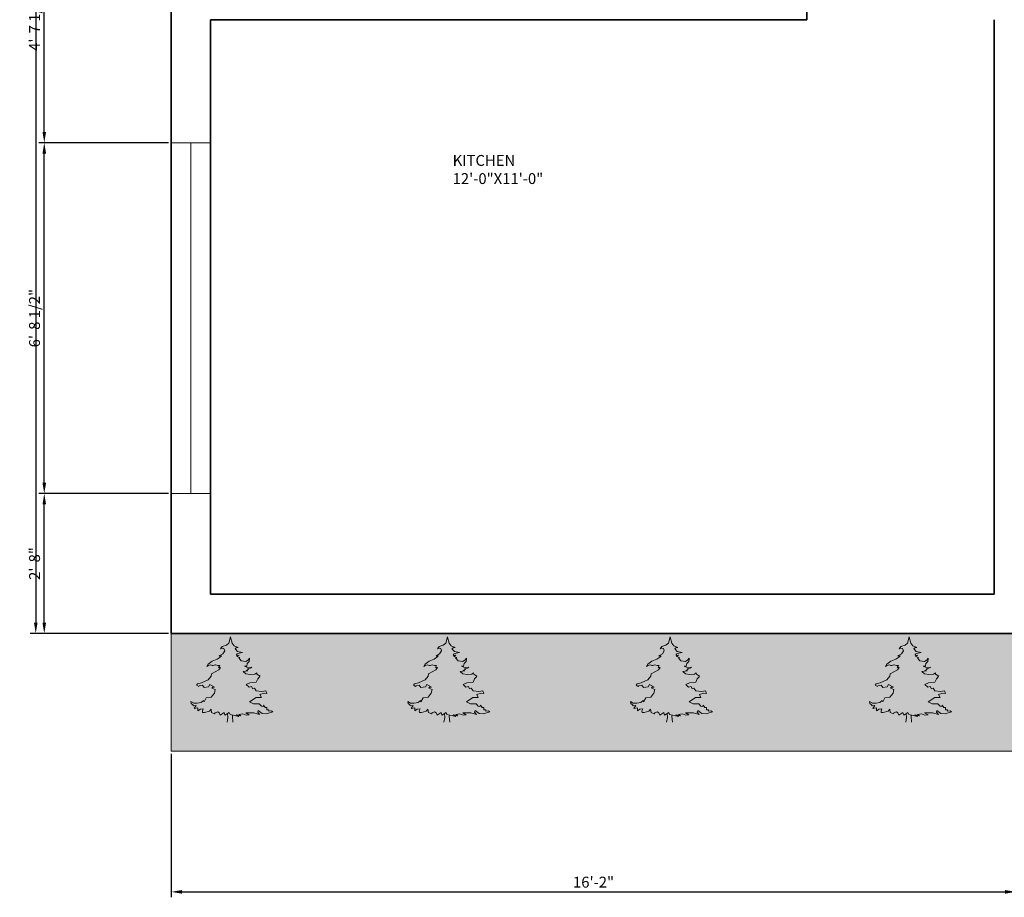
# Model space of a CAD drawing. Units: inches. Extents: x 2981 to 3526, y 1512 to 2158.
# Tile 1 of 4: x 2981 to 3207, y 1512 to 1713. Entities that reach past the tile are written whole.
import ezdxf

# ---------------------------------------------------------------- set-up
doc = ezdxf.new("R2010")
doc.units = ezdxf.units.IN
for name, color, linetype, lineweight in [('A-ANNO-DIMS', 2, 'Continuous', 18), ('A-AREA-IDEN', 7, 'Continuous', 18), ('A-GLAZ', 4, 'Continuous', 18), ('A-WALL', 7, 'Continuous', 35), ('L-GRND-PATT', 8, 'Continuous', 13), ('L-PLNT', 3, 'Continuous', 18), ('L-PLNT-BEDS', 7, 'Continuous', 18)]:
    doc.layers.add(name, color=color, linetype=linetype, lineweight=lineweight)
doc.layers.add('L-PLNT-PATT', color=116, linetype='Continuous', lineweight=13, true_color=0x136734)
doc.styles.get("Standard").update_dxf_attribs({"font": 'arial.ttf'})
doc.dimstyles.new('ISO-25', dxfattribs={"dimtxt": 2.5, "dimasz": 2.5, "dimexe": 1.25, "dimexo": 0.625, "dimtad": 1, "dimlunit": 3, "dimtxsty": 'Standard', "dimcen": 2.5, "dimadec": 0, "dimazin": 0, "dimtfac": 1, "dimtmove": 0, "dimatfit": 3, "dimfxl": 1, "dimarcsym": 0})

# ---------------------------------------------------------------- blocks, each defined once
blk = doc.blocks.new('*U13')
for p, q in [((-9.75, 0), (-8.263, 7.598)), ((-8.263, 7.598), (-8.747, 14.105)), ((-0.771, 9.56), (-0.69, 11.833)), ((0, 0), (-0.771, 9.56))]:
    blk.add_line(p, q)
for points in [[(-3.9, 142.35), (-6.596, 132.037), (-10.801, 128.443), (-17.81, 126.047), (-20.614, 122.452), (-17.81, 123.65), (-15.007, 123.051), (-13.605, 118.858), (-16.876, 114.065), (-21.549, 111.07), (-22.951, 109.872), (-19.212, 110.471), (-19.68, 109.273), (-26.222, 105.079), (-34.633, 101.485), (-41.175, 96.693), (-43.511, 93.098), (-41.175, 94.296), (-36.969, 95.494), (-34.633, 94.296), (-32.764, 94.296), (-29.493, 95.494)], [(-3.759, 141.97), (-1.074, 131.643), (2.437, 127.141), (8.84, 124.493), (6.568, 124.493), (4.09, 123.169), (4.296, 121.846), (7.807, 117.874), (16.069, 116.02), (10.492, 115.226), (5.535, 113.372), (6.981, 112.843), (5.948, 110.989), (10.286, 112.048), (6.775, 109.401), (11.732, 108.077), (9.873, 107.282), (13.797, 102.516), (21.852, 101.192), (25.983, 103.84), (28.048, 106.488), (27.842, 105.164), (27.429, 101.457), (24.124, 97.75), (23.091, 93.513), (19.58, 93.513), (23.505, 91.66), (28.255, 90.866), (31.973, 91.925), (29.081, 89.806), (24.537, 88.747), (26.809, 88.218), (22.472, 86.099), (24.95, 85.57), (17.308, 84.246), (21.852, 80.804), (29.081, 79.215), (36.723, 80.009), (39.821, 82.392), (40.028, 80.009), (45.398, 76.567)], [(-29.25, 95.55), (-25.287, 94.296), (-22.016, 94.296), (-23.885, 91.301), (-20.614, 91.301), (-23.418, 87.108), (-35.567, 80.518), (-36.035, 76.924), (-41.175, 70.334), (-52.389, 65.542), (-58.931, 63.744), (-60.8, 61.348), (-57.062, 59.551), (-56.128, 60.749), (-50.987, 61.348), (-48.184, 57.754), (-40.707, 58.952), (-38.371, 62.546), (-30.427, 58.353), (-33.698, 58.353), (-35.1, 56.556), (-29.493, 54.159), (-30.894, 48.169), (-36.035, 41.579), (-44.446, 40.381), (-48.184, 33.791), (-49.118, 36.188), (-52.857, 32.593), (-59.399, 31.395), (-65.473, 31.395), (-70.146, 34.39), (-69.679, 30.796), (-66.875, 28.999), (-65.941, 27.202), (-61.268, 27.801), (-64.539, 22.409), (-58.464, 23.607), (-58.464, 18.815), (-54.258, 21.211), (-49.586, 21.81), (-50.987, 18.815), (-50.52, 15.82), (-47.249, 15.82), (-39.306, 18.216), (-36.502, 21.211), (-35.567, 15.82), (-30.427, 13.423), (-29.493, 15.221), (-25.287, 17.018), (-22.951, 15.221), (-21.081, 11.626), (-14.539, 15.82), (-13.138, 11.626), (-6.128, 15.82), (-4.726, 12.824), (10.226, 9.23), (5.554, 12.225), (13.497, 10.428), (10.226, 12.824), (16.768, 13.423), (22.376, 11.626), (27.516, 12.225), (21.909, 15.221), (34.993, 15.221), (44.806, 12.824), (41.535, 16.419), (42.469, 19.414), (49.011, 14.023), (56.487, 13.423), (66.768, 17.018), (64.431, 18.815), (60.226, 18.216), (60.226, 20.612), (56.955, 20.612), (56.955, 24.206), (54.151, 24.206), (51.348, 28.4), (50.413, 26.004), (47.609, 26.603), (43.871, 30.197), (38.731, 30.197), (34.525, 30.197), (27.983, 33.791), (38.731, 40.98), (47.609, 40.98), (45.273, 45.773), (52.282, 48.169), (56.955, 47.57), (55.086, 52.362), (48.544, 51.164), (39.198, 52.362), (35.927, 56.556), (33.123, 55.357), (31.254, 59.551), (27.049, 58.353), (22.376, 62.546), (28.451, 65.542), (39.198, 66.74), (41.535, 72.131), (45.273, 76.325)]]:
    blk.add_lwpolyline(points)
blk = doc.blocks.new('*D15')
at = {"layer": 'A-ANNO-DIMS', "color": 0, "lineweight": -2, "transparency": 16777216}
for p, q in [((3014.77, 2112.2), (2983.05, 2112.2)), ((2984.3, 2109.7), (2984.3, 1574.7)), ((3014.77, 1572.2), (2983.05, 1572.2))]:
    blk.add_line(p, q, dxfattribs=at)
at = {"layer": 'A-ANNO-DIMS', "color": 0, "transparency": 16777216}
for points in [[(2983.89, 2109.7), (2984.72, 2109.7), (2984.3, 2112.2)], [(2983.89, 1574.7), (2984.72, 1574.7), (2984.3, 1572.2)]]:
    blk.add_solid(points, dxfattribs=at)
at = {"layer": 'Defpoints', "color": 0, "transparency": 16777216}
for p in [(3015.4, 2112.2), (2984.3, 1572.2), (3015.4, 1572.2)]:
    blk.add_point(p, dxfattribs=at)
at = {"layer": 'A-ANNO-DIMS', "color": 0, "transparency": 16777216, "insert": (2982.41, 1842.2), "char_height": 2.5, "attachment_point": 5, "rotation": 90}
blk.add_mtext("45'", dxfattribs=at)
blk = doc.blocks.new('*D40')
at = {"layer": 'A-ANNO-DIMS', "color": 0, "lineweight": -2, "transparency": 16777216}
for p, q in [((3015.4, 1544.58), (3015.4, 1511.59)), ((3209.4, 1544.58), (3209.4, 1511.59)), ((3017.9, 1512.84), (3206.9, 1512.84))]:
    blk.add_line(p, q, dxfattribs=at)
at = {"layer": 'A-ANNO-DIMS', "color": 0, "transparency": 16777216}
for points in [[(3017.9, 1513.26), (3017.9, 1512.43), (3015.4, 1512.84)], [(3206.9, 1513.26), (3206.9, 1512.43), (3209.4, 1512.84)]]:
    blk.add_solid(points, dxfattribs=at)
at = {"layer": 'Defpoints', "color": 0, "transparency": 16777216}
for p in [(3015.4, 1545.2), (3209.4, 1545.2), (3209.4, 1512.84)]:
    blk.add_point(p, dxfattribs=at)
at = {"layer": 'A-ANNO-DIMS', "color": 0, "transparency": 16777216, "insert": (3112.4, 1514.75), "char_height": 2.5, "attachment_point": 5}
blk.add_mtext('16\'-2"', dxfattribs=at)
blk = doc.blocks.new('*D44')
at = {"layer": 'A-ANNO-DIMS', "color": 0, "lineweight": -2, "transparency": 16777216}
for p, q in [((3014.77, 1684.94), (2985, 1684.94)), ((2986.25, 1606.84), (2986.25, 1682.44)), ((3014.77, 1604.34), (2985, 1604.34))]:
    blk.add_line(p, q, dxfattribs=at)
at = {"layer": 'A-ANNO-DIMS', "color": 0, "transparency": 16777216}
for points in [[(2985.84, 1682.44), (2986.67, 1682.44), (2986.25, 1684.94)], [(2985.84, 1606.84), (2986.67, 1606.84), (2986.25, 1604.34)]]:
    blk.add_solid(points, dxfattribs=at)
at = {"layer": 'Defpoints', "color": 0, "transparency": 16777216}
for p in [(2986.25, 1684.94), (3015.4, 1684.94), (3015.4, 1604.34)]:
    blk.add_point(p, dxfattribs=at)
at = {"layer": 'A-ANNO-DIMS', "color": 0, "transparency": 16777216, "insert": (2984.34, 1644.64), "char_height": 2.5, "attachment_point": 5, "rotation": 90}
blk.add_mtext('6\'-8 1/2"', dxfattribs=at)
blk = doc.blocks.new('*D45')
at = {"layer": 'A-ANNO-DIMS', "color": 0, "lineweight": -2, "transparency": 16777216}
for p, q in [((3014.77, 1604.34), (2985, 1604.34)), ((2986.25, 1574.7), (2986.25, 1601.84)), ((3014.77, 1572.2), (2985, 1572.2))]:
    blk.add_line(p, q, dxfattribs=at)
at = {"layer": 'A-ANNO-DIMS', "color": 0, "transparency": 16777216}
for points in [[(2985.84, 1601.84), (2986.67, 1601.84), (2986.25, 1604.34)], [(2985.84, 1574.7), (2986.67, 1574.7), (2986.25, 1572.2)]]:
    blk.add_solid(points, dxfattribs=at)
at = {"layer": 'Defpoints', "color": 0, "transparency": 16777216}
for p in [(2986.25, 1604.34), (3015.4, 1604.34), (3015.4, 1572.2)]:
    blk.add_point(p, dxfattribs=at)
at = {"layer": 'A-ANNO-DIMS', "color": 0, "transparency": 16777216, "insert": (2984.35, 1588.27), "char_height": 2.5, "attachment_point": 5, "rotation": 90}
blk.add_mtext('2\'-8"', dxfattribs=at)
blk = doc.blocks.new('*D51')
at = {"layer": 'A-ANNO-DIMS', "color": 0, "lineweight": -2, "transparency": 16777216}
for p, q in [((3014.77, 1740.56), (2985, 1740.56)), ((2986.25, 1687.44), (2986.25, 1738.06)), ((3014.77, 1684.94), (2985, 1684.94))]:
    blk.add_line(p, q, dxfattribs=at)
at = {"layer": 'A-ANNO-DIMS', "color": 0, "transparency": 16777216}
for points in [[(2985.84, 1738.06), (2986.67, 1738.06), (2986.25, 1740.56)], [(2985.84, 1687.44), (2986.67, 1687.44), (2986.25, 1684.94)]]:
    blk.add_solid(points, dxfattribs=at)
at = {"layer": 'Defpoints', "color": 0, "transparency": 16777216}
for p in [(2986.25, 1740.56), (3015.4, 1740.56), (3015.4, 1684.94)]:
    blk.add_point(p, dxfattribs=at)
at = {"layer": 'A-ANNO-DIMS', "color": 0, "transparency": 16777216, "insert": (2984.34, 1712.75), "char_height": 2.5, "attachment_point": 5, "rotation": 90}
blk.add_mtext('4\'-7 1/2"', dxfattribs=at)

msp = doc.modelspace()

# ---------------------------------------------------------------- hatches: boundary and pattern name
at = {"layer": 'L-GRND-PATT'}
h = msp.add_hatch(color=256, dxfattribs=at)
h.dxf.hatch_style = 1
h.paths.add_polyline_path([(3209.399, 1563.202), (3209.399, 1572.202), (3015.399, 1572.202), (3015.399, 1545.202), (3209.399, 1545.202), (3209.399, 1554.202)])
h.paths.add_polyline_path([(3038.736, 1554.203), (3037.324, 1553.709), (3036.297, 1553.792), (3035.398, 1554.532), (3035.27, 1554.121), (3035.719, 1553.627), (3034.371, 1553.956), (3032.573, 1553.956), (3033.344, 1553.545), (3032.638, 1553.462), (3031.867, 1553.709), (3030.968, 1553.627), (3031.418, 1553.298), (3030.327, 1553.545), (3030.968, 1553.133), (3028.914, 1553.627), (3028.722, 1554.039), (3027.759, 1553.462), (3027.566, 1554.039), (3026.668, 1553.462), (3026.411, 1553.956), (3026.09, 1554.203), (3025.512, 1553.956), (3025.384, 1553.709), (3024.677, 1554.039), (3024.549, 1554.779), (3024.164, 1554.368), (3023.073, 1554.039), (3022.623, 1554.039), (3022.559, 1554.45), (3022.752, 1554.861), (3022.11, 1554.779), (3021.532, 1554.45), (3021.532, 1555.108), (3020.697, 1554.944), (3021.147, 1555.684), (3020.505, 1555.602), (3020.376, 1555.849), (3019.991, 1556.096), (3019.927, 1556.59), (3020.569, 1556.178), (3021.403, 1556.178), (3022.302, 1556.343), (3022.816, 1556.837), (3022.944, 1556.507), (3023.458, 1557.413), (3024.613, 1557.577), (3025.319, 1558.483), (3025.512, 1559.306), (3024.742, 1559.635), (3024.934, 1559.882), (3025.384, 1559.882), (3024.292, 1560.458), (3023.971, 1559.964), (3022.944, 1559.799), (3022.559, 1560.293), (3021.853, 1560.211), (3021.724, 1560.046), (3021.211, 1560.293), (3021.468, 1560.622), (3022.366, 1560.869), (3023.907, 1561.528), (3024.613, 1562.433), (3024.677, 1562.927), (3026.346, 1563.832), (3026.732, 1564.408), (3026.282, 1564.408), (3026.539, 1564.82), (3026.09, 1564.82), (3025.539, 1564.994), (3024.913, 1564.765), (3024.485, 1564.984), (3023.907, 1564.82), (3023.586, 1564.655), (3023.907, 1565.149), (3024.806, 1565.807), (3025.961, 1566.301), (3026.86, 1566.877), (3026.924, 1567.042), (3026.411, 1566.959), (3026.603, 1567.124), (3027.245, 1567.535), (3027.695, 1568.194), (3027.502, 1568.77), (3027.117, 1568.852), (3026.732, 1568.688), (3027.117, 1569.181), (3028.08, 1569.511), (3028.657, 1570.004), (3029.031, 1571.432), (3029.416, 1569.95), (3029.898, 1569.332), (3030.778, 1568.968), (3030.466, 1568.968), (3030.126, 1568.786), (3030.154, 1568.604), (3030.636, 1568.059), (3031.771, 1567.804), (3031.005, 1567.695), (3030.324, 1567.44), (3030.523, 1567.368), (3030.381, 1567.113), (3030.977, 1567.258), (3030.494, 1566.895), (3031.175, 1566.713), (3030.92, 1566.604), (3031.459, 1565.949), (3032.566, 1565.767), (3033.133, 1566.131), (3033.417, 1566.494), (3033.389, 1566.313), (3033.332, 1565.803), (3032.878, 1565.294), (3032.736, 1564.712), (3032.254, 1564.712), (3032.793, 1564.457), (3033.445, 1564.348), (3033.956, 1564.494), (3033.559, 1564.203), (3032.935, 1564.057), (3033.247, 1563.985), (3032.651, 1563.693), (3032.991, 1563.621), (3031.941, 1563.439), (3032.566, 1562.966), (3033.559, 1562.748), (3034.609, 1562.857), (3035.034, 1563.184), (3035.063, 1562.857), (3035.808, 1562.379), (3035.27, 1561.775), (3034.949, 1561.034), (3033.472, 1560.869), (3032.638, 1560.458), (3033.28, 1559.882), (3033.857, 1560.046), (3034.114, 1559.47), (3034.499, 1559.635), (3034.949, 1559.059), (3036.233, 1558.894), (3037.131, 1559.059), (3037.388, 1558.4), (3036.746, 1558.483), (3035.783, 1558.153), (3036.104, 1557.495), (3034.884, 1557.495), (3033.408, 1556.507), (3034.307, 1556.014), (3034.884, 1556.014), (3035.591, 1556.014), (3036.104, 1555.52), (3036.489, 1555.438), (3036.618, 1555.767), (3037.003, 1555.191), (3037.388, 1555.191), (3037.388, 1554.697), (3037.837, 1554.697), (3037.837, 1554.368), (3038.415, 1554.45)], flags=16)
h.paths.add_polyline_path([(3069.74, 1556.59), (3070.382, 1556.178), (3071.217, 1556.178), (3072.115, 1556.343), (3072.629, 1556.837), (3072.757, 1556.507), (3073.271, 1557.413), (3074.426, 1557.577), (3075.133, 1558.483), (3075.325, 1559.306), (3074.555, 1559.635), (3074.747, 1559.882), (3075.197, 1559.882), (3074.105, 1560.458), (3073.785, 1559.964), (3072.757, 1559.799), (3072.372, 1560.293), (3071.666, 1560.211), (3071.538, 1560.046), (3071.024, 1560.293), (3071.281, 1560.622), (3072.18, 1560.869), (3073.72, 1561.528), (3074.426, 1562.433), (3074.491, 1562.927), (3076.16, 1563.832), (3076.545, 1564.408), (3076.096, 1564.408), (3076.352, 1564.82), (3075.903, 1564.82), (3075.352, 1564.994), (3074.726, 1564.765), (3074.298, 1564.984), (3073.72, 1564.82), (3073.399, 1564.655), (3073.72, 1565.149), (3074.619, 1565.807), (3075.774, 1566.301), (3076.673, 1566.877), (3076.737, 1567.042), (3076.224, 1566.959), (3076.416, 1567.124), (3077.058, 1567.535), (3077.508, 1568.194), (3077.315, 1568.77), (3076.93, 1568.852), (3076.545, 1568.688), (3076.93, 1569.181), (3077.893, 1569.511), (3078.471, 1570.004), (3078.844, 1571.432), (3079.229, 1569.95), (3079.712, 1569.332), (3080.591, 1568.968), (3080.279, 1568.968), (3079.939, 1568.786), (3079.967, 1568.604), (3080.449, 1568.059), (3081.584, 1567.804), (3080.818, 1567.695), (3080.137, 1567.44), (3080.336, 1567.368), (3080.194, 1567.113), (3080.79, 1567.258), (3080.308, 1566.895), (3080.989, 1566.713), (3080.733, 1566.604), (3081.272, 1565.949), (3082.379, 1565.767), (3082.946, 1566.131), (3083.23, 1566.494), (3083.202, 1566.313), (3083.145, 1565.803), (3082.691, 1565.294), (3082.549, 1564.712), (3082.067, 1564.712), (3082.606, 1564.457), (3083.258, 1564.348), (3083.769, 1564.494), (3083.372, 1564.203), (3082.748, 1564.057), (3083.06, 1563.985), (3082.464, 1563.693), (3082.804, 1563.621), (3081.755, 1563.439), (3082.379, 1562.966), (3083.372, 1562.748), (3084.422, 1562.857), (3084.847, 1563.184), (3084.876, 1562.857), (3085.622, 1562.379), (3085.083, 1561.775), (3084.762, 1561.034), (3083.285, 1560.869), (3082.451, 1560.458), (3083.093, 1559.882), (3083.67, 1560.046), (3083.927, 1559.47), (3084.312, 1559.635), (3084.762, 1559.059), (3086.046, 1558.894), (3086.945, 1559.059), (3087.201, 1558.4), (3086.559, 1558.483), (3085.596, 1558.153), (3085.917, 1557.495), (3084.698, 1557.495), (3083.221, 1556.507), (3084.12, 1556.014), (3084.698, 1556.014), (3085.404, 1556.014), (3085.917, 1555.52), (3086.303, 1555.438), (3086.431, 1555.767), (3086.816, 1555.191), (3087.201, 1555.191), (3087.201, 1554.697), (3087.651, 1554.697), (3087.651, 1554.368), (3088.228, 1554.45), (3088.549, 1554.203), (3087.137, 1553.709), (3086.11, 1553.792), (3085.211, 1554.532), (3085.083, 1554.121), (3085.532, 1553.627), (3084.184, 1553.956), (3082.387, 1553.956), (3083.157, 1553.545), (3082.451, 1553.462), (3081.68, 1553.709), (3080.782, 1553.627), (3081.231, 1553.298), (3080.14, 1553.545), (3080.782, 1553.133), (3078.728, 1553.627), (3078.535, 1554.039), (3077.572, 1553.462), (3077.379, 1554.039), (3076.481, 1553.462), (3076.224, 1553.956), (3075.903, 1554.203), (3075.325, 1553.956), (3075.197, 1553.709), (3074.491, 1554.039), (3074.362, 1554.779), (3073.977, 1554.368), (3072.886, 1554.039), (3072.436, 1554.039), (3072.372, 1554.45), (3072.565, 1554.861), (3071.923, 1554.779), (3071.345, 1554.45), (3071.345, 1555.108), (3070.51, 1554.944), (3070.96, 1555.684), (3070.318, 1555.602), (3070.19, 1555.849), (3069.804, 1556.096)], flags=16)
h.paths.add_polyline_path([(3120.884, 1556.59), (3121.526, 1556.178), (3122.361, 1556.178), (3123.259, 1556.343), (3123.773, 1556.837), (3123.901, 1556.507), (3124.415, 1557.413), (3125.57, 1557.577), (3126.277, 1558.483), (3126.469, 1559.306), (3125.699, 1559.635), (3125.891, 1559.882), (3126.341, 1559.882), (3125.249, 1560.458), (3124.928, 1559.964), (3123.901, 1559.799), (3123.516, 1560.293), (3122.81, 1560.211), (3122.682, 1560.046), (3122.168, 1560.293), (3122.425, 1560.622), (3123.324, 1560.869), (3124.864, 1561.528), (3125.57, 1562.433), (3125.635, 1562.927), (3127.304, 1563.832), (3127.689, 1564.408), (3127.239, 1564.408), (3127.496, 1564.82), (3127.047, 1564.82), (3126.496, 1564.994), (3125.87, 1564.765), (3125.442, 1564.984), (3124.864, 1564.82), (3124.543, 1564.655), (3124.864, 1565.149), (3125.763, 1565.807), (3126.918, 1566.301), (3127.817, 1566.877), (3127.881, 1567.042), (3127.368, 1566.959), (3127.56, 1567.124), (3128.202, 1567.535), (3128.652, 1568.194), (3128.459, 1568.77), (3128.074, 1568.852), (3127.689, 1568.688), (3128.074, 1569.181), (3129.037, 1569.511), (3129.615, 1570.004), (3129.988, 1571.432), (3130.373, 1569.95), (3130.856, 1569.332), (3131.735, 1568.968), (3131.423, 1568.968), (3131.083, 1568.786), (3131.111, 1568.604), (3131.593, 1568.059), (3132.728, 1567.804), (3131.962, 1567.695), (3131.281, 1567.44), (3131.48, 1567.368), (3131.338, 1567.113), (3131.934, 1567.258), (3131.452, 1566.895), (3132.133, 1566.713), (3131.877, 1566.604), (3132.416, 1565.949), (3133.523, 1565.767), (3134.09, 1566.131), (3134.374, 1566.494), (3134.346, 1566.313), (3134.289, 1565.803), (3133.835, 1565.294), (3133.693, 1564.712), (3133.211, 1564.712), (3133.75, 1564.457), (3134.402, 1564.348), (3134.913, 1564.494), (3134.516, 1564.203), (3133.892, 1564.057), (3134.204, 1563.985), (3133.608, 1563.693), (3133.948, 1563.621), (3132.899, 1563.439), (3133.523, 1562.966), (3134.516, 1562.748), (3135.566, 1562.857), (3135.991, 1563.184), (3136.02, 1562.857), (3136.765, 1562.379), (3136.227, 1561.775), (3135.906, 1561.034), (3134.429, 1560.869), (3133.595, 1560.458), (3134.237, 1559.882), (3134.814, 1560.046), (3135.071, 1559.47), (3135.456, 1559.635), (3135.906, 1559.059), (3137.19, 1558.894), (3138.088, 1559.059), (3138.345, 1558.4), (3137.703, 1558.483), (3136.74, 1558.153), (3137.061, 1557.495), (3135.842, 1557.495), (3134.365, 1556.507), (3135.264, 1556.014), (3135.842, 1556.014), (3136.548, 1556.014), (3137.061, 1555.52), (3137.446, 1555.438), (3137.575, 1555.767), (3137.96, 1555.191), (3138.345, 1555.191), (3138.345, 1554.697), (3138.795, 1554.697), (3138.795, 1554.368), (3139.372, 1554.45), (3139.693, 1554.203), (3138.281, 1553.709), (3137.254, 1553.792), (3136.355, 1554.532), (3136.227, 1554.121), (3136.676, 1553.627), (3135.328, 1553.956), (3133.531, 1553.956), (3134.301, 1553.545), (3133.595, 1553.462), (3132.824, 1553.709), (3131.926, 1553.627), (3132.375, 1553.298), (3131.284, 1553.545), (3131.926, 1553.133), (3129.872, 1553.627), (3129.679, 1554.039), (3128.716, 1553.462), (3128.523, 1554.039), (3127.625, 1553.462), (3127.368, 1553.956), (3127.047, 1554.203), (3126.469, 1553.956), (3126.341, 1553.709), (3125.635, 1554.039), (3125.506, 1554.779), (3125.121, 1554.368), (3124.03, 1554.039), (3123.58, 1554.039), (3123.516, 1554.45), (3123.709, 1554.861), (3123.067, 1554.779), (3122.489, 1554.45), (3122.489, 1555.108), (3121.654, 1554.944), (3122.104, 1555.684), (3121.462, 1555.602), (3121.334, 1555.849), (3120.948, 1556.096)], flags=16)
h.paths.add_polyline_path([(3175.793, 1556.59), (3176.435, 1556.178), (3177.27, 1556.178), (3178.169, 1556.343), (3178.682, 1556.837), (3178.811, 1556.507), (3179.324, 1557.413), (3180.48, 1557.577), (3181.186, 1558.483), (3181.378, 1559.306), (3180.608, 1559.635), (3180.801, 1559.882), (3181.25, 1559.882), (3180.159, 1560.458), (3179.838, 1559.964), (3178.811, 1559.799), (3178.425, 1560.293), (3177.719, 1560.211), (3177.591, 1560.046), (3177.077, 1560.293), (3177.334, 1560.622), (3178.233, 1560.869), (3179.773, 1561.528), (3180.48, 1562.433), (3180.544, 1562.927), (3182.213, 1563.832), (3182.598, 1564.408), (3182.149, 1564.408), (3182.406, 1564.82), (3181.956, 1564.82), (3181.405, 1564.994), (3180.779, 1564.765), (3180.351, 1564.984), (3179.773, 1564.82), (3179.453, 1564.655), (3179.773, 1565.149), (3180.672, 1565.807), (3181.828, 1566.301), (3182.726, 1566.877), (3182.791, 1567.042), (3182.277, 1566.959), (3182.47, 1567.124), (3183.112, 1567.535), (3183.561, 1568.194), (3183.368, 1568.77), (3182.983, 1568.852), (3182.598, 1568.688), (3182.983, 1569.181), (3183.946, 1569.511), (3184.524, 1570.004), (3184.897, 1571.432), (3185.283, 1569.95), (3185.765, 1569.332), (3186.645, 1568.968), (3186.332, 1568.968), (3185.992, 1568.786), (3186.02, 1568.604), (3186.503, 1568.059), (3187.638, 1567.804), (3186.871, 1567.695), (3186.19, 1567.44), (3186.389, 1567.368), (3186.247, 1567.113), (3186.843, 1567.258), (3186.361, 1566.895), (3187.042, 1566.713), (3186.786, 1566.604), (3187.325, 1565.949), (3188.432, 1565.767), (3189, 1566.131), (3189.283, 1566.494), (3189.255, 1566.313), (3189.198, 1565.803), (3188.744, 1565.294), (3188.602, 1564.712), (3188.12, 1564.712), (3188.659, 1564.457), (3189.312, 1564.348), (3189.823, 1564.494), (3189.425, 1564.203), (3188.801, 1564.057), (3189.113, 1563.985), (3188.517, 1563.693), (3188.858, 1563.621), (3187.808, 1563.439), (3188.432, 1562.966), (3189.425, 1562.748), (3190.475, 1562.857), (3190.901, 1563.184), (3190.929, 1562.857), (3191.675, 1562.379), (3191.136, 1561.775), (3190.815, 1561.034), (3189.339, 1560.869), (3188.504, 1560.458), (3189.146, 1559.882), (3189.724, 1560.046), (3189.98, 1559.47), (3190.366, 1559.635), (3190.815, 1559.059), (3192.099, 1558.894), (3192.998, 1559.059), (3193.255, 1558.4), (3192.613, 1558.483), (3191.65, 1558.153), (3191.971, 1557.495), (3190.751, 1557.495), (3189.274, 1556.507), (3190.173, 1556.014), (3190.751, 1556.014), (3191.457, 1556.014), (3191.971, 1555.52), (3192.356, 1555.438), (3192.484, 1555.767), (3192.869, 1555.191), (3193.255, 1555.191), (3193.255, 1554.697), (3193.704, 1554.697), (3193.704, 1554.368), (3194.282, 1554.45), (3194.603, 1554.203), (3193.19, 1553.709), (3192.163, 1553.792), (3191.264, 1554.532), (3191.136, 1554.121), (3191.586, 1553.627), (3190.237, 1553.956), (3188.44, 1553.956), (3189.21, 1553.545), (3188.504, 1553.462), (3187.734, 1553.709), (3186.835, 1553.627), (3187.284, 1553.298), (3186.193, 1553.545), (3186.835, 1553.133), (3184.781, 1553.627), (3184.588, 1554.039), (3183.625, 1553.462), (3183.433, 1554.039), (3182.534, 1553.462), (3182.277, 1553.956), (3181.956, 1554.203), (3181.378, 1553.956), (3181.25, 1553.709), (3180.544, 1554.039), (3180.415, 1554.779), (3180.03, 1554.368), (3178.939, 1554.039), (3178.49, 1554.039), (3178.425, 1554.45), (3178.618, 1554.861), (3177.976, 1554.779), (3177.398, 1554.45), (3177.398, 1555.108), (3176.564, 1554.944), (3177.013, 1555.684), (3176.371, 1555.602), (3176.243, 1555.849), (3175.858, 1556.096)], flags=16)
at = {"layer": 'L-PLNT-PATT'}
h = msp.add_hatch(color=256, dxfattribs=at)
h.dxf.hatch_style = 1
h.paths.add_polyline_path([(3035.808, 1562.379), (3035.063, 1562.857), (3035.034, 1563.184), (3034.609, 1562.857), (3033.559, 1562.748), (3032.566, 1562.966), (3031.941, 1563.439), (3032.991, 1563.621), (3032.651, 1563.693), (3033.247, 1563.985), (3032.935, 1564.057), (3033.559, 1564.203), (3033.956, 1564.494), (3033.445, 1564.348), (3032.793, 1564.457), (3032.254, 1564.712), (3032.736, 1564.712), (3032.878, 1565.294), (3033.332, 1565.803), (3033.407, 1566.482), (3033.133, 1566.131), (3032.566, 1565.767), (3031.459, 1565.949), (3030.92, 1566.604), (3031.175, 1566.713), (3030.494, 1566.895), (3030.977, 1567.258), (3030.381, 1567.113), (3030.523, 1567.368), (3030.324, 1567.44), (3031.005, 1567.695), (3031.771, 1567.804), (3030.636, 1568.059), (3030.036, 1568.738), (3030.602, 1569.041), (3029.898, 1569.332), (3029.416, 1569.95), (3029.031, 1571.432), (3028.657, 1570.004), (3028.08, 1569.511), (3027.117, 1569.181), (3026.732, 1568.688), (3027.117, 1568.852), (3027.502, 1568.77), (3027.695, 1568.194), (3027.245, 1567.535), (3026.603, 1567.124), (3026.411, 1566.959), (3026.924, 1567.042), (3026.86, 1566.877), (3025.961, 1566.301), (3024.806, 1565.807), (3023.907, 1565.149), (3023.586, 1564.655), (3023.907, 1564.82), (3024.485, 1564.984), (3024.806, 1564.82), (3025.063, 1564.82), (3025.539, 1564.994), (3026.09, 1564.82), (3026.539, 1564.82), (3026.282, 1564.408), (3026.732, 1564.408), (3026.346, 1563.832), (3024.677, 1562.927), (3024.613, 1562.433), (3023.907, 1561.528), (3022.366, 1560.869), (3021.468, 1560.622), (3021.211, 1560.293), (3021.724, 1560.046), (3021.853, 1560.211), (3022.559, 1560.293), (3022.944, 1559.799), (3023.971, 1559.964), (3024.292, 1560.458), (3025.384, 1559.882), (3024.934, 1559.882), (3024.742, 1559.635), (3025.512, 1559.306), (3025.319, 1558.483), (3024.613, 1557.577), (3023.458, 1557.413), (3022.944, 1556.507), (3022.816, 1556.837), (3022.302, 1556.343), (3021.403, 1556.178), (3020.569, 1556.178), (3019.927, 1556.59), (3019.991, 1556.096), (3020.376, 1555.849), (3020.505, 1555.602), (3021.147, 1555.684), (3020.697, 1554.944), (3021.532, 1555.108), (3021.532, 1554.45), (3022.11, 1554.779), (3022.752, 1554.861), (3022.559, 1554.45), (3022.623, 1554.039), (3023.073, 1554.039), (3024.164, 1554.368), (3024.549, 1554.779), (3024.677, 1554.039), (3025.384, 1553.709), (3025.512, 1553.956), (3026.09, 1554.203), (3026.411, 1553.956), (3026.668, 1553.462), (3027.566, 1554.039), (3027.759, 1553.462), (3028.722, 1554.039), (3028.914, 1553.627), (3030.968, 1553.133), (3030.327, 1553.545), (3031.418, 1553.298), (3030.968, 1553.627), (3031.867, 1553.709), (3032.638, 1553.462), (3033.344, 1553.545), (3032.573, 1553.956), (3034.371, 1553.956), (3035.719, 1553.627), (3035.27, 1554.121), (3035.398, 1554.532), (3036.297, 1553.792), (3037.324, 1553.709), (3038.736, 1554.203), (3038.415, 1554.45), (3037.837, 1554.368), (3037.837, 1554.697), (3037.388, 1554.697), (3037.388, 1555.191), (3037.003, 1555.191), (3036.618, 1555.767), (3036.489, 1555.438), (3036.104, 1555.52), (3035.591, 1556.014), (3034.884, 1556.014), (3034.307, 1556.014), (3033.408, 1556.507), (3034.884, 1557.495), (3036.104, 1557.495), (3035.783, 1558.153), (3036.746, 1558.483), (3037.388, 1558.4), (3037.131, 1559.059), (3036.233, 1558.894), (3034.949, 1559.059), (3034.499, 1559.635), (3034.114, 1559.47), (3033.857, 1560.046), (3033.28, 1559.882), (3032.638, 1560.458), (3033.472, 1560.869), (3034.949, 1561.034), (3035.27, 1561.775)])
h.paths.add_polyline_path([(3084.312, 1559.635), (3083.927, 1559.47), (3083.67, 1560.046), (3083.093, 1559.882), (3082.451, 1560.458), (3083.285, 1560.869), (3084.762, 1561.034), (3085.083, 1561.775), (3085.622, 1562.379), (3084.876, 1562.857), (3084.847, 1563.184), (3084.422, 1562.857), (3083.372, 1562.748), (3082.379, 1562.966), (3081.755, 1563.439), (3082.804, 1563.621), (3082.464, 1563.693), (3083.06, 1563.985), (3082.748, 1564.057), (3083.372, 1564.203), (3083.769, 1564.494), (3083.258, 1564.348), (3082.606, 1564.457), (3082.067, 1564.712), (3082.549, 1564.712), (3082.691, 1565.294), (3083.145, 1565.803), (3083.221, 1566.482), (3082.946, 1566.131), (3082.379, 1565.767), (3081.272, 1565.949), (3080.733, 1566.604), (3080.989, 1566.713), (3080.308, 1566.895), (3080.79, 1567.258), (3080.194, 1567.113), (3080.336, 1567.368), (3080.137, 1567.44), (3080.818, 1567.695), (3081.584, 1567.804), (3080.449, 1568.059), (3079.849, 1568.738), (3080.415, 1569.041), (3079.712, 1569.332), (3079.229, 1569.95), (3078.844, 1571.432), (3078.471, 1570.004), (3077.893, 1569.511), (3076.93, 1569.181), (3076.545, 1568.688), (3076.93, 1568.852), (3077.315, 1568.77), (3077.508, 1568.194), (3077.058, 1567.535), (3076.416, 1567.124), (3076.224, 1566.959), (3076.737, 1567.042), (3076.673, 1566.877), (3075.774, 1566.301), (3074.619, 1565.807), (3073.72, 1565.149), (3073.399, 1564.655), (3073.72, 1564.82), (3074.298, 1564.984), (3074.619, 1564.82), (3074.876, 1564.82), (3075.352, 1564.994), (3075.903, 1564.82), (3076.352, 1564.82), (3076.096, 1564.408), (3076.545, 1564.408), (3076.16, 1563.832), (3074.491, 1562.927), (3074.426, 1562.433), (3073.72, 1561.528), (3072.18, 1560.869), (3071.281, 1560.622), (3071.024, 1560.293), (3071.538, 1560.046), (3071.666, 1560.211), (3072.372, 1560.293), (3072.757, 1559.799), (3073.785, 1559.964), (3074.105, 1560.458), (3075.197, 1559.882), (3074.747, 1559.882), (3074.555, 1559.635), (3075.325, 1559.306), (3075.133, 1558.483), (3074.426, 1557.577), (3073.271, 1557.413), (3072.757, 1556.507), (3072.629, 1556.837), (3072.115, 1556.343), (3071.217, 1556.178), (3070.382, 1556.178), (3069.74, 1556.59), (3069.804, 1556.096), (3070.19, 1555.849), (3070.318, 1555.602), (3070.96, 1555.684), (3070.51, 1554.944), (3071.345, 1555.108), (3071.345, 1554.45), (3071.923, 1554.779), (3072.565, 1554.861), (3072.372, 1554.45), (3072.436, 1554.039), (3072.886, 1554.039), (3073.977, 1554.368), (3074.362, 1554.779), (3074.491, 1554.039), (3075.197, 1553.709), (3075.325, 1553.956), (3075.903, 1554.203), (3076.224, 1553.956), (3076.481, 1553.462), (3077.379, 1554.039), (3077.572, 1553.462), (3078.535, 1554.039), (3078.728, 1553.627), (3080.782, 1553.133), (3080.14, 1553.545), (3081.231, 1553.298), (3080.782, 1553.627), (3081.68, 1553.709), (3082.451, 1553.462), (3083.157, 1553.545), (3082.387, 1553.956), (3084.184, 1553.956), (3085.532, 1553.627), (3085.083, 1554.121), (3085.211, 1554.532), (3086.11, 1553.792), (3087.137, 1553.709), (3088.549, 1554.203), (3088.228, 1554.45), (3087.651, 1554.368), (3087.651, 1554.697), (3087.201, 1554.697), (3087.201, 1555.191), (3086.816, 1555.191), (3086.431, 1555.767), (3086.303, 1555.438), (3085.917, 1555.52), (3085.404, 1556.014), (3084.698, 1556.014), (3084.12, 1556.014), (3083.221, 1556.507), (3084.698, 1557.495), (3085.917, 1557.495), (3085.596, 1558.153), (3086.559, 1558.483), (3087.201, 1558.4), (3086.945, 1559.059), (3086.046, 1558.894), (3084.762, 1559.059)])
h.paths.add_polyline_path([(3135.842, 1557.495), (3137.061, 1557.495), (3136.74, 1558.153), (3137.703, 1558.483), (3138.345, 1558.4), (3138.088, 1559.059), (3137.19, 1558.894), (3135.906, 1559.059), (3135.456, 1559.635), (3135.071, 1559.47), (3134.814, 1560.046), (3134.237, 1559.882), (3133.595, 1560.458), (3134.429, 1560.869), (3135.906, 1561.034), (3136.227, 1561.775), (3136.765, 1562.379), (3136.02, 1562.857), (3135.991, 1563.184), (3135.566, 1562.857), (3134.516, 1562.748), (3133.523, 1562.966), (3132.899, 1563.439), (3133.948, 1563.621), (3133.608, 1563.693), (3134.204, 1563.985), (3133.892, 1564.057), (3134.516, 1564.203), (3134.913, 1564.494), (3134.402, 1564.348), (3133.75, 1564.457), (3133.211, 1564.712), (3133.693, 1564.712), (3133.835, 1565.294), (3134.289, 1565.803), (3134.365, 1566.482), (3134.09, 1566.131), (3133.523, 1565.767), (3132.416, 1565.949), (3131.877, 1566.604), (3132.133, 1566.713), (3131.452, 1566.895), (3131.934, 1567.258), (3131.338, 1567.113), (3131.48, 1567.368), (3131.281, 1567.44), (3131.962, 1567.695), (3132.728, 1567.804), (3131.593, 1568.059), (3130.993, 1568.738), (3131.559, 1569.041), (3130.856, 1569.332), (3130.373, 1569.95), (3129.988, 1571.432), (3129.615, 1570.004), (3129.037, 1569.511), (3128.074, 1569.181), (3127.689, 1568.688), (3128.074, 1568.852), (3128.459, 1568.77), (3128.652, 1568.194), (3128.202, 1567.535), (3127.56, 1567.124), (3127.368, 1566.959), (3127.881, 1567.042), (3127.817, 1566.877), (3126.918, 1566.301), (3125.763, 1565.807), (3124.864, 1565.149), (3124.543, 1564.655), (3124.864, 1564.82), (3125.442, 1564.984), (3125.763, 1564.82), (3126.02, 1564.82), (3126.496, 1564.994), (3127.047, 1564.82), (3127.496, 1564.82), (3127.239, 1564.408), (3127.689, 1564.408), (3127.304, 1563.832), (3125.635, 1562.927), (3125.57, 1562.433), (3124.864, 1561.528), (3123.324, 1560.869), (3122.425, 1560.622), (3122.168, 1560.293), (3122.682, 1560.046), (3122.81, 1560.211), (3123.516, 1560.293), (3123.901, 1559.799), (3124.928, 1559.964), (3125.249, 1560.458), (3126.341, 1559.882), (3125.891, 1559.882), (3125.699, 1559.635), (3126.469, 1559.306), (3126.277, 1558.483), (3125.57, 1557.577), (3124.415, 1557.413), (3123.901, 1556.507), (3123.773, 1556.837), (3123.259, 1556.343), (3122.361, 1556.178), (3121.526, 1556.178), (3120.884, 1556.59), (3120.948, 1556.096), (3121.334, 1555.849), (3121.462, 1555.602), (3122.104, 1555.684), (3121.654, 1554.944), (3122.489, 1555.108), (3122.489, 1554.45), (3123.067, 1554.779), (3123.709, 1554.861), (3123.516, 1554.45), (3123.58, 1554.039), (3124.03, 1554.039), (3125.121, 1554.368), (3125.506, 1554.779), (3125.635, 1554.039), (3126.341, 1553.709), (3126.469, 1553.956), (3127.047, 1554.203), (3127.368, 1553.956), (3127.625, 1553.462), (3128.523, 1554.039), (3128.716, 1553.462), (3129.679, 1554.039), (3129.872, 1553.627), (3131.926, 1553.133), (3131.284, 1553.545), (3132.375, 1553.298), (3131.926, 1553.627), (3132.824, 1553.709), (3133.595, 1553.462), (3134.301, 1553.545), (3133.531, 1553.956), (3135.328, 1553.956), (3136.676, 1553.627), (3136.227, 1554.121), (3136.355, 1554.532), (3137.254, 1553.792), (3138.281, 1553.709), (3139.693, 1554.203), (3139.372, 1554.45), (3138.795, 1554.368), (3138.795, 1554.697), (3138.345, 1554.697), (3138.345, 1555.191), (3137.96, 1555.191), (3137.575, 1555.767), (3137.446, 1555.438), (3137.061, 1555.52), (3136.548, 1556.014), (3135.842, 1556.014), (3135.264, 1556.014), (3134.365, 1556.507)])
h.paths.add_polyline_path([(3192.998, 1559.059), (3192.099, 1558.894), (3190.815, 1559.059), (3190.366, 1559.635), (3189.98, 1559.47), (3189.724, 1560.046), (3189.146, 1559.882), (3188.504, 1560.458), (3189.339, 1560.869), (3190.815, 1561.034), (3191.136, 1561.775), (3191.675, 1562.379), (3190.929, 1562.857), (3190.901, 1563.184), (3190.475, 1562.857), (3189.425, 1562.748), (3188.432, 1562.966), (3187.808, 1563.439), (3188.858, 1563.621), (3188.517, 1563.693), (3189.113, 1563.985), (3188.801, 1564.057), (3189.425, 1564.203), (3189.823, 1564.494), (3189.312, 1564.348), (3188.659, 1564.457), (3188.12, 1564.712), (3188.602, 1564.712), (3188.744, 1565.294), (3189.198, 1565.803), (3189.274, 1566.482), (3189, 1566.131), (3188.432, 1565.767), (3187.325, 1565.949), (3186.786, 1566.604), (3187.042, 1566.713), (3186.361, 1566.895), (3186.843, 1567.258), (3186.247, 1567.113), (3186.389, 1567.368), (3186.19, 1567.44), (3186.871, 1567.695), (3187.638, 1567.804), (3186.503, 1568.059), (3185.902, 1568.738), (3186.469, 1569.041), (3185.765, 1569.332), (3185.283, 1569.95), (3184.897, 1571.432), (3184.524, 1570.004), (3183.946, 1569.511), (3182.983, 1569.181), (3182.598, 1568.688), (3182.983, 1568.852), (3183.368, 1568.77), (3183.561, 1568.194), (3183.112, 1567.535), (3182.47, 1567.124), (3182.277, 1566.959), (3182.791, 1567.042), (3182.726, 1566.877), (3181.828, 1566.301), (3180.672, 1565.807), (3179.773, 1565.149), (3179.453, 1564.655), (3179.773, 1564.82), (3180.351, 1564.984), (3180.672, 1564.82), (3180.929, 1564.82), (3181.405, 1564.994), (3181.956, 1564.82), (3182.406, 1564.82), (3182.149, 1564.408), (3182.598, 1564.408), (3182.213, 1563.832), (3180.544, 1562.927), (3180.48, 1562.433), (3179.773, 1561.528), (3178.233, 1560.869), (3177.334, 1560.622), (3177.077, 1560.293), (3177.591, 1560.046), (3177.719, 1560.211), (3178.425, 1560.293), (3178.811, 1559.799), (3179.838, 1559.964), (3180.159, 1560.458), (3181.25, 1559.882), (3180.801, 1559.882), (3180.608, 1559.635), (3181.378, 1559.306), (3181.186, 1558.483), (3180.48, 1557.577), (3179.324, 1557.413), (3178.811, 1556.507), (3178.682, 1556.837), (3178.169, 1556.343), (3177.27, 1556.178), (3176.435, 1556.178), (3175.793, 1556.59), (3175.858, 1556.096), (3176.243, 1555.849), (3176.371, 1555.602), (3177.013, 1555.684), (3176.564, 1554.944), (3177.398, 1555.108), (3177.398, 1554.45), (3177.976, 1554.779), (3178.618, 1554.861), (3178.425, 1554.45), (3178.49, 1554.039), (3178.939, 1554.039), (3180.03, 1554.368), (3180.415, 1554.779), (3180.544, 1554.039), (3181.25, 1553.709), (3181.378, 1553.956), (3181.956, 1554.203), (3182.277, 1553.956), (3182.534, 1553.462), (3183.433, 1554.039), (3183.625, 1553.462), (3184.588, 1554.039), (3184.781, 1553.627), (3186.835, 1553.133), (3186.193, 1553.545), (3187.284, 1553.298), (3186.835, 1553.627), (3187.734, 1553.709), (3188.504, 1553.462), (3189.21, 1553.545), (3188.44, 1553.956), (3190.237, 1553.956), (3191.586, 1553.627), (3191.136, 1554.121), (3191.264, 1554.532), (3192.163, 1553.792), (3193.19, 1553.709), (3194.603, 1554.203), (3194.282, 1554.45), (3193.704, 1554.368), (3193.704, 1554.697), (3193.255, 1554.697), (3193.255, 1555.191), (3192.869, 1555.191), (3192.484, 1555.767), (3192.356, 1555.438), (3191.971, 1555.52), (3191.457, 1556.014), (3190.751, 1556.014), (3190.173, 1556.014), (3189.274, 1556.507), (3190.751, 1557.495), (3191.971, 1557.495), (3191.65, 1558.153), (3192.613, 1558.483), (3193.255, 1558.4)])

# ---------------------------------------------------------------- linework, layer by layer
at = {"layer": 'A-GLAZ'}
for p, q in [((3024.399, 1684.94), (3015.399, 1684.94)), ((3015.399, 1684.94), (3015.399, 1604.339)), ((3024.399, 1684.94), (3019.899, 1684.94)), ((3019.899, 1684.94), (3019.899, 1604.339)), ((3024.399, 1604.339), (3024.399, 1684.94)), ((3015.399, 1604.339), (3024.399, 1604.339))]:
    msp.add_line(p, q, dxfattribs=at)
at = {"layer": 'A-WALL'}
for p, q in [((3015.399, 1572.202), (3015.399, 2112.202)), ((3161.399, 1713.202), (3161.399, 1795.202)), ((3024.399, 1581.202), (3024.399, 1713.202)), ((3161.399, 1713.202), (3024.399, 1713.202)), ((3204.399, 1581.202), (3204.399, 1713.202)), ((3204.399, 1661.202), (3204.399, 1656.202)), ((3204.399, 1581.202), (3024.399, 1581.202)), ((3495.399, 1572.202), (3015.399, 1572.202))]:
    msp.add_line(p, q, dxfattribs=at)
at = {"layer": 'L-PLNT-BEDS'}
for p, q in [((3015.399, 1545.202), (3015.399, 1572.202)), ((3209.399, 1545.202), (3015.399, 1545.202))]:
    msp.add_line(p, q, dxfattribs=at)

# ---------------------------------------------------------------- block references
at = {"layer": 'L-PLNT', "xscale": 0.13737964736475, "yscale": 0.13737964736475, "zscale": 0.13737964736475}
for p in [(3029.564, 1551.865), (3079.377, 1551.865), (3130.521, 1551.865), (3185.43, 1551.865)]:
    msp.add_blockref('*U13', p, dxfattribs=at)

# ---------------------------------------------------------------- texts
at = {"layer": 'A-AREA-IDEN', "insert": (3080.039, 1682.117), "char_height": 2.5, "attachment_point": 1}
msp.add_mtext_dynamic_manual_height_columns('KITCHEN\\P12\'-0"X11\'-0"', width=124.36038, gutter_width=12.5, heights=[0], dxfattribs=at)

# ---------------------------------------------------------------- dimensions: what is measured, and where the dimension line sits
at = {"layer": 'A-ANNO-DIMS'}
for base, p1, p2, override, picture, middle in [((2984.303, 1572.202), (3015.399, 2112.202), (3015.399, 1572.202), {"dimclrd": 0, "dimclre": 0, "dimclrt": 0}, '*D15', (2982.407, 1842.202)), ((2986.254, 1740.564), (3015.399, 1684.94), (3015.399, 1740.564), {"dimdec": 1, "dimlfac": 1, "dimrnd": 0, "dimzin": 1, "dimdsep": 46, "dimlunit": 4, "dimfrac": 2}, '*D51', (2984.337, 1712.752)), ((2986.254, 1684.94), (3015.399, 1604.339), (3015.399, 1684.94), {"dimdec": 1, "dimlfac": 1, "dimrnd": 0, "dimzin": 1, "dimdsep": 46, "dimlunit": 4, "dimfrac": 2}, '*D44', (2984.337, 1644.64)), ((2986.254, 1604.339), (3015.399, 1572.202), (3015.399, 1604.339), {"dimdec": 1, "dimlfac": 1, "dimrnd": 0, "dimzin": 1, "dimdsep": 46, "dimlunit": 4, "dimfrac": 2}, '*D45', (2984.353, 1588.271))]:
    dim = msp.add_linear_dim(base=base, p1=p1, p2=p2, angle=90, dimstyle='ISO-25', override=override, dxfattribs=at)
    dim.commit()
    dim.dimension.update_dxf_attribs({"geometry": picture, "text_midpoint": middle})
dim = msp.add_linear_dim(base=(3209.399, 1512.844), p1=(3015.399, 1545.202), p2=(3209.399, 1545.202), dimstyle='ISO-25', override={"dimdec": 1, "dimlfac": 1, "dimrnd": 0, "dimzin": 1, "dimdsep": 46, "dimlunit": 4, "dimfrac": 2}, dxfattribs=at)
dim.commit()
dim.dimension.update_dxf_attribs({"geometry": '*D40', "text_midpoint": (3112.399, 1514.746)})

doc.saveas('drawing.dxf')
